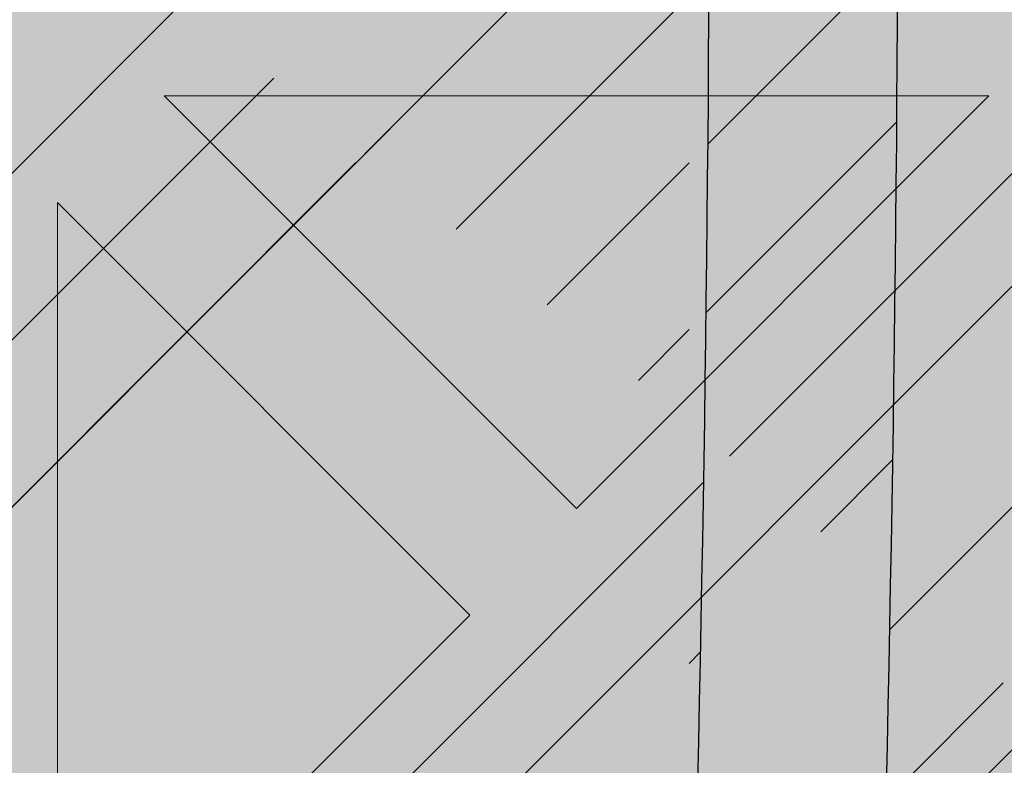
# Model space of a CAD drawing. Units: inches. Extents: x 844 to 2234, y 346 to 1084.
# Tile 11 of 93: x 1122.921 to 1124.585, y 692.442 to 693.702. Entities that reach past the tile are written whole.
import ezdxf

# ---------------------------------------------------------------- set-up
doc = ezdxf.new("R2010")
doc.units = ezdxf.units.IN
doc.header["$MEASUREMENT"] = 0
for name, color, linetype, lineweight in [('A-ANNO-DIMS', 2, 'Continuous', 18), ('furniture', 8, 'Continuous', 18), ('RA-AP-01$0$INT', 35, 'Continuous', 5)]:
    doc.layers.add(name, color=color, linetype=linetype, lineweight=lineweight)
doc.layers.add('RA-AP-01$0$FURN', color=3, linetype='Continuous')
doc.layers.add('RA-AP-01$0$WOOD', color=64, linetype='Continuous')
doc.styles.get("Standard").update_dxf_attribs({"font": 'arial.ttf'})
doc.dimstyles.get("Standard").update_dxf_attribs({"dimtxt": 6, "dimasz": 3, "dimexe": 0.18, "dimexo": 0.0625, "dimgap": 0.09, "dimtad": 0, "dimtih": 1, "dimtoh": 1, "dimdec": 1, "dimzin": 0, "dimdsep": 46, "dimlunit": 3, "dimtxsty": 'Standard', "dimblk": 'ARCHTICK', "dimcen": 0.09, "dimadec": 0, "dimazin": 0, "dimtfac": 1, "dimtdec": 1, "dimtofl": 0, "dimtmove": 0, "dimatfit": 3, "dimfxl": 1, "dimtolj": 1, "dimtzin": 0, "dimarcsym": 0})

# ---------------------------------------------------------------- blocks, each defined once
blk = doc.blocks.new('A$C18D01794')
at = {"layer": 'RA-AP-01$0$INT'}
h = blk.add_hatch(color=256, dxfattribs=at)
h.paths.add_polyline_path([(4.585917135068449, -6.356712009588271), (4.555206456959269, -6.35671200958746), (4.555206456959137, -6.387422687716308), (4.874495778835233, -6.706712009592356), (4.90520645695423, -6.676001331474049)])
h.paths.add_polyline_path([(5.255206456948813, -6.387422687716306), (5.255206456948682, -6.356712009605972), (5.224495778822613, -6.356712009605161), (4.905206456953498, -6.676001331474273), (4.935917135072151, -6.706712009592924)])
h.paths.add_polyline_path([(4.935917135072559, -6.706712009592068), (4.905206456953564, -6.737422687710376), (5.255206456951813, -7.087422687708613), (5.255206456951549, -7.026001331471008)])
h.paths.add_polyline_path([(4.555206456956399, -7.026001331471013), (4.555206456956134, -7.087422687708616), (4.905206456953821, -6.737422687710943), (4.874495778835166, -6.70671200959229)])
h = blk.add_hatch(color=256, dxfattribs=at)
h.paths.add_polyline_path([(4.585917135068448, -6.356712009588273), (4.614201406330596, -6.356712009589021), (4.668846067270487, -6.411356670531338), (4.723490728212344, -6.356712009591912), (4.771774999457151, -6.35671200959319), (4.826419660396886, -6.411356670535356), (4.862780050090322, -6.374996280843536), (4.844495778842715, -6.356712009595112), (4.862780050090411, -6.356712009595595), (4.905206456960182, -6.399138416468211), (4.947632863832445, -6.356712009597838), (4.965917135079675, -6.356712009598322), (4.947632863831759, -6.374996280845421), (4.983993253523576, -6.411356670538857), (5.038637914464627, -6.356712009600247), (5.08692218571208, -6.356712009601523), (5.141566846649976, -6.411356670541852), (5.196211507589851, -6.356712009604411), (5.224495778822615, -6.356712009605161), (4.905206456953975, -6.676001331473793)])
h.paths.add_polyline_path([(4.895206456956031, -6.637717060225675), (4.895206456958921, -6.528427738347902), (4.840561796018589, -6.583072399285802)], flags=16)
h.paths.add_polyline_path([(4.915206456955638, -6.637717060226121), (4.969851117895509, -6.583072399288678), (4.915206456957609, -6.528427738348344)], flags=16)
h.paths.add_polyline_path([(4.826419660395175, -6.568930263661755), (4.881064321335613, -6.514285602723745), (4.771774999456703, -6.514285602720857)], flags=16)
h.paths.add_polyline_path([(4.983993253519558, -6.568930263665262), (5.038637914460456, -6.514285602726792), (4.929348592581548, -6.514285602724816)], flags=16)
h.paths.add_polyline_path([(4.881064321336025, -6.494285602723742), (4.826419660397532, -6.439640941782821), (4.771774999457062, -6.494285602720859)], flags=16)
h.paths.add_polyline_path([(4.929348592582019, -6.494285602724817), (5.038637914460982, -6.494285602726792), (4.983993253522945, -6.439640941786327)], flags=16)
h.paths.add_polyline_path([(4.895206456960191, -6.480143467100443), (4.895206456962115, -6.407422687715913), (4.876922185715016, -6.389138416467584), (4.840561796021581, -6.425498806159401)], flags=16)
h.paths.add_polyline_path([(4.915206456958487, -6.480143467100889), (4.969851117899527, -6.425498806162279), (4.933490728206909, -6.389138416468043), (4.9152064569598, -6.40742268771434)], flags=16)
h.paths.add_polyline_path([(4.757632863832376, -6.480143467096812), (4.812277524772842, -6.425498806158772), (4.757632863834348, -6.370854145217844)], flags=16)
h.paths.add_polyline_path([(4.737632863832376, -6.480143467096286), (4.737632863834348, -6.370854145217375), (4.682988202893906, -6.425498806155385)], flags=16)
h.paths.add_polyline_path([(5.05278005008503, -6.480143467103376), (5.052780050087917, -6.370854145224413), (4.998135389146995, -6.425498806162908)], flags=16)
h.paths.add_polyline_path([(5.072780050085024, -6.480143467103744), (5.127424711025931, -6.42549880616527), (5.072780050087916, -6.370854145224832)], flags=16)
h.paths.add_polyline_path([(4.935917135072783, -6.706712009592292), (5.255206456948811, -6.387422687716309), (5.255206456948932, -6.415706958964177), (5.200561796010279, -6.470351619902839), (5.255206456949403, -6.524996280841948), (5.25520645694961, -6.5732805520894), (5.200561796009787, -6.627925213029239), (5.236922185702417, -6.664285602721864), (5.255206456949919, -6.646001331474357), (5.255206456949998, -6.664285602721898), (5.212780050078687, -6.706712009592262), (5.25520645695036, -6.749138416463932), (5.255206456950438, -6.767422687711313), (5.236922185702424, -6.749138416463297), (5.200561796009796, -6.785498806155928), (5.255206456950753, -6.840143467096874), (5.25520645695096, -6.888427738341682), (5.200561796010322, -6.943072399282328), (5.255206456951428, -6.997717060223427), (5.255206456951547, -7.026001331471006)])
h.paths.add_polyline_path([(5.042988202883395, -6.785498806155427), (5.097632863823085, -6.840143467095101), (5.097632863822622, -6.730854145216193)], flags=16)
h.paths.add_polyline_path([(5.028846067259663, -6.771356670531693), (5.083490728198774, -6.716712009592573), (4.974201406321001, -6.716712009593042)], flags=16)
h.paths.add_polyline_path([(5.117632863823087, -6.840143467095186), (5.172277524762331, -6.785498806155926), (5.11763286382262, -6.730854145216225)], flags=16)
h.paths.add_polyline_path([(5.08349072819877, -6.696712009593886), (5.028846067259652, -6.642067348654775), (4.974201406320998, -6.696712009593438)], flags=16)
h.paths.add_polyline_path([(5.131774999446817, -6.854285602718917), (5.186419660386065, -6.799640941779662), (5.241064321325782, -6.854285602719365)], flags=17)
h.paths.add_polyline_path([(5.131774999446228, -6.716712009592374), (5.186419660386065, -6.771356670532194), (5.222780050079488, -6.734996280838764), (5.204495778832781, -6.716712009592063)], flags=16)
h.paths.add_polyline_path([(5.097632863822613, -6.682569873970264), (5.097632863823061, -6.573280552091354), (5.042988202883383, -6.627925213031044)], flags=16)
h.paths.add_polyline_path([(5.131774999446899, -6.874285602718915), (5.241064321325809, -6.874285602719364), (5.186419660386591, -6.928930263658598)], flags=17)
h.paths.add_polyline_path([(5.131774999446226, -6.696712009594078), (5.204495778830767, -6.696712009594374), (5.22278005007868, -6.67842773834687), (5.186419660386049, -6.642067348654249)], flags=16)
h.paths.add_polyline_path([(5.11763286382262, -6.682569873970225), (5.17227752476232, -6.627925213030515), (5.117632863823064, -6.573280552091267)], flags=16)
h.paths.add_polyline_path([(5.186419660386069, -6.613783077405491), (5.241064321325754, -6.559138416465795), (5.131774999446791, -6.559138416466263)], flags=16)
h.paths.add_polyline_path([(5.131774999446872, -6.539138416466263), (5.24106432132578, -6.539138416465794), (5.186419660386554, -6.484493755526573)], flags=16)
h.paths.add_polyline_path([(5.255206456951811, -7.08742268770861), (5.255206456951895, -7.106712009588038), (4.555206456956052, -7.106712009588038), (4.555206456956136, -7.087422687708617), (4.905206456953973, -6.737422687710788)])
h.paths.add_polyline_path([(4.983993253513404, -6.8444937555241), (4.92934859257295, -6.899138416462108), (5.03863791445186, -6.899138416465014)], flags=16)
h.paths.add_polyline_path([(4.969851117889988, -6.83035161990006), (4.915206456952556, -6.775706958960171), (4.915206456949648, -6.884996280837944)], flags=16)
h.paths.add_polyline_path([(4.929348592572535, -6.919138416462105), (4.983993253511019, -6.973783077403037), (5.038637914451496, -6.919138416465012)], flags=16)
h.paths.add_polyline_path([(5.052780050074912, -6.93328055208906), (4.998135389134438, -6.987925213027088), (5.052780050072919, -7.042569873968025)], flags=16)
h.paths.add_polyline_path([(5.07278005007491, -6.933280552089588), (5.072780050072918, -7.042569873968497), (5.127424711013374, -6.987925213030498)], flags=16)
h.paths.add_polyline_path([(4.89520645695295, -6.775706958959721), (4.840561796013067, -6.830351619897157), (4.895206456950961, -6.884996280837494)], flags=16)
h.paths.add_polyline_path([(4.915206456948365, -6.933280552085403), (4.915206456946434, -7.006001331471951), (4.933490728192729, -7.024285602719066), (4.969851117886972, -6.987925213026453)], flags=16)
h.paths.add_polyline_path([(4.881064321327021, -6.899138416461022), (4.82641966038902, -6.84449375552057), (4.771774999448108, -6.899138416459029)], flags=16)
h.paths.add_polyline_path([(4.895206456950073, -6.933280552084951), (4.840561796009022, -6.987925213023558), (4.876922185700835, -7.024285602716997), (4.895206456948749, -7.006001331469487)], flags=16)
h.paths.add_polyline_path([(4.983993253510392, -7.0020673486505), (4.947632863816944, -7.038427738342319), (4.965917135064043, -7.05671200959023), (5.038637914448995, -7.056712009591555)], flags=16)
h.paths.add_polyline_path([(4.881064321326543, -6.91913841646102), (4.771774999447578, -6.919138416459031), (4.826419660385607, -6.973783077399508)], flags=16)
h.paths.add_polyline_path([(4.905206456946447, -7.014285602717636), (4.862780050074785, -7.056712009588352), (4.947632863816685, -7.056712009589775)], flags=16)
h.paths.add_polyline_path([(5.14156684663679, -7.002067348654549), (5.086922185696452, -7.056712009592438), (5.196211507574223, -7.056712009594425)], flags=16)
h.paths.add_polyline_path([(4.8264196603837, -7.002067348646972), (4.771774999442643, -7.056712009585575), (4.8444957788276, -7.056712009587508), (4.862780050075511, -7.038427738340416)], flags=16)
h.paths.add_polyline_path([(4.812277524760289, -6.98792521302292), (4.757632863822258, -6.933280552082447), (4.757632863819352, -7.042569873961408)], flags=16)
h.paths.add_polyline_path([(4.73763286382226, -6.933280552082079), (4.682988202881349, -6.987925213020536), (4.737632863819352, -7.04256987396099)], flags=16)
h.paths.add_polyline_path([(4.723490728195188, -7.056712009584289), (4.668846067257299, -7.002067348643949), (4.614201406317417, -7.056712009581383)], flags=16)
h.paths.add_polyline_path([(4.597632863829262, -6.706712009592262), (4.555206456957951, -6.664285602721896), (4.555206456958029, -6.646001331474357), (4.573490728205535, -6.664285602721864), (4.609851117898167, -6.627925213029238), (4.555206456958338, -6.573280552089402), (4.555206456958546, -6.524996280841952), (4.60985111789767, -6.470351619902839), (4.555206456959015, -6.415706958964177), (4.555206456959138, -6.387422687716309), (4.874495778835167, -6.70671200959229), (4.5552064569564, -7.026001331471015), (4.555206456956523, -6.997717060223433), (4.609851117897629, -6.94307239928233), (4.555206456956988, -6.888427738341681), (4.555206456957198, -6.840143467096881), (4.609851117898153, -6.78549880615593), (4.573490728205528, -6.749138416463297), (4.555206456957507, -6.76742268771132), (4.555206456957585, -6.749138416463933)])
h.paths.add_polyline_path([(4.712780050085332, -6.730854145216195), (4.712780050084863, -6.840143467095105), (4.767424711024555, -6.785498806155427)], flags=16)
h.paths.add_polyline_path([(4.726922185709173, -6.716712009592573), (4.781566846648288, -6.771356670531693), (4.836211507586949, -6.716712009593043)], flags=16)
h.paths.add_polyline_path([(4.692780050085327, -6.730854145216225), (4.638135389145619, -6.785498806155928), (4.692780050084865, -6.840143467095185)], flags=16)
h.paths.add_polyline_path([(4.726922185709182, -6.696712009593886), (4.836211507586949, -6.696712009593436), (4.7815668466483, -6.642067348654773)], flags=16)
h.paths.add_polyline_path([(4.678637914461726, -6.71671200959237), (4.605917135075169, -6.716712009592063), (4.587632863828464, -6.734996280838766), (4.623993253521887, -6.771356670532195)], flags=16)
h.paths.add_polyline_path([(4.712780050085336, -6.68256987397026), (4.767424711024568, -6.627925213031042), (4.71278005008489, -6.573280552091352)], flags=16)
h.paths.add_polyline_path([(4.678637914461726, -6.696712009594076), (4.623993253521899, -6.642067348654247), (4.587632863829271, -6.67842773834687), (4.605917135077185, -6.696712009594376)], flags=16)
h.paths.add_polyline_path([(4.692780050085336, -6.682569873970228), (4.692780050084889, -6.573280552091267), (4.638135389145632, -6.627925213030515)], flags=16)
h.paths.add_polyline_path([(4.623993253521885, -6.799640941779662), (4.678637914461131, -6.854285602718915), (4.56934859258217, -6.854285602719365)], flags=17)
h.paths.add_polyline_path([(4.623993253521901, -6.613783077405509), (4.678637914461158, -6.559138416466263), (4.569348592582195, -6.559138416465795)], flags=16)
h.paths.add_polyline_path([(4.678637914461051, -6.874285602718915), (4.623993253521361, -6.928930263658598), (4.569348592582143, -6.874285602719364)], flags=17)
h.paths.add_polyline_path([(4.678637914461076, -6.539138416466263), (4.623993253521399, -6.484493755526573), (4.569348592582167, -6.539138416465796)], flags=16)
h = blk.add_hatch(color=256, dxfattribs=at)
h.paths.add_polyline_path([(4.895206456952951, -6.77570695895972), (4.840561796013068, -6.830351619897156), (4.895206456950958, -6.884996280837495)])
h.paths.add_polyline_path([(4.915206456949649, -6.884996280837942), (4.969851117889987, -6.830351619900054), (4.915206456952556, -6.775706958960171)])
h.paths.add_polyline_path([(5.038637914451862, -6.899138416465013), (4.983993253513403, -6.8444937555241), (4.929348592572953, -6.899138416462106)])
h.paths.add_polyline_path([(4.929348592572535, -6.919138416462105), (4.983993253511018, -6.973783077403037), (5.038637914451497, -6.919138416465012)])
h.paths.add_polyline_path([(4.915206456948366, -6.933280552085397), (4.915206456946433, -7.006001331471951), (4.93349072819273, -7.024285602719068), (4.969851117886972, -6.987925213026454)])
h.paths.add_polyline_path([(5.038637914448995, -7.056712009591553), (4.983993253510389, -7.002067348650502), (4.947632863816946, -7.038427738342318), (4.965917135064043, -7.05671200959023)])
h.paths.add_polyline_path([(5.05278005007292, -7.042569873968023), (5.05278005007491, -6.933280552089059), (4.998135389134438, -6.987925213027088)])
h.paths.add_polyline_path([(5.07278005007292, -7.042569873968496), (5.127424711013374, -6.987925213030498), (5.072780050074909, -6.933280552089588)])
h.paths.add_polyline_path([(5.141566846636789, -7.002067348654547), (5.086922185696449, -7.056712009592438), (5.196211507574223, -7.056712009594425)])
h.paths.add_polyline_path([(4.947632863816688, -7.056712009589774), (4.905206456946449, -7.014285602717634), (4.862780050074784, -7.056712009588353)])
h.paths.add_polyline_path([(4.840561796009025, -6.987925213023556), (4.876922185700834, -7.024285602716997), (4.895206456948747, -7.006001331469488), (4.895206456950075, -6.933280552084953)])
h.paths.add_polyline_path([(4.88106432132654, -6.919138416461021), (4.771774999447577, -6.919138416459031), (4.826419660385606, -6.973783077399508)])
h.paths.add_polyline_path([(4.881064321327019, -6.899138416461022), (4.826419660389019, -6.844493755520571), (4.771774999448108, -6.89913841645903)])
h.paths.add_polyline_path([(4.757632863819352, -7.042569873961409), (4.812277524760284, -6.987925213022922), (4.757632863822259, -6.933280552082447)])
h.paths.add_polyline_path([(4.8264196603837, -7.002067348646974), (4.771774999442646, -7.056712009585575), (4.844495778827599, -7.05671200958751), (4.862780050075512, -7.038427738340417)])
h.paths.add_polyline_path([(4.737632863819352, -7.042569873960988), (4.737632863822258, -6.933280552082078), (4.682988202881349, -6.987925213020538)])
h.paths.add_polyline_path([(4.668846067257299, -7.002067348643952), (4.61420140631742, -7.056712009581384), (4.723490728195189, -7.056712009584292)])
for p, q in [((4.935917135072783, -6.706712009592292), (5.255206456951548, -7.026001331471007)), ((4.905206456953975, -6.737422687710788), (5.255206456951811, -7.087422687708611)), ((4.915206456952556, -6.775706958960171), (4.969851117889986, -6.830351619900053)), ((4.915206456949648, -6.884996280837942), (4.915206456952556, -6.775706958960171)), ((4.915206456949651, -6.88499628083794), (4.969851117889986, -6.830351619900053)), ((4.929348592572952, -6.899138416462106), (4.983993253513403, -6.844493755524101)), ((4.983993253513404, -6.844493755524103), (5.038637914451862, -6.899138416465012)), ((5.038637914451862, -6.899138416465012), (4.929348592572952, -6.899138416462106))]:
    blk.add_line(p, q, dxfattribs=at)
blk = doc.blocks.new('A$C32926AE1')
at = {"layer": 'RA-AP-01$0$FURN'}
h = blk.add_hatch(dxfattribs=at)
h.set_pattern_fill('ANSI31', color=256, scale=0.1, style=0)
h.set_pattern_definition([(45, (0, 0), (-0.0088388347648318, 0.0088388347648318), [])])
edge = h.paths.add_edge_path(flags=16)
edge.add_arc((4.904771284329206, 4.246793130718756), 0.2603971832811541, 75.22398030683196, 104.7760196931204)
edge.add_arc((4.904771284329206, 4.246793130718756), 0.2603971832811541, 75.223980306832, 104.77601969312039, ccw=False)
edge = h.paths.add_edge_path(flags=16)
edge.add_arc((4.904771284329206, 4.067062675376612), 0.2603971832811541, 255.2239803068796, 284.776019693168)
edge.add_arc((4.904771284329206, 4.067062675376612), 0.2603971832811541, 255.22398030687958, 284.77601969316805, ccw=False)
edge = h.paths.add_edge_path(flags=0)
edge.add_arc((4.904771284329206, 4.067062675376612), 0.2603971832811541, 255.2239803068796, 284.776019693168)
edge.add_arc((4.904771284329206, 4.067062675376612), 0.2603971832811541, 255.22398030687958, 284.77601969316805, ccw=False)
edge = h.paths.add_edge_path(flags=0)
edge.add_arc((4.904771284329206, 4.067062675376612), 0.2603971832811541, 255.2239803068796, 284.776019693168)
edge.add_arc((4.904771284329206, 4.067062675376612), 0.2603971832811541, 255.22398030687958, 284.77601969316805, ccw=False)
edge = h.paths.add_edge_path()
edge.add_arc((4.604388392048174, 4.588829985554312), 0.1599999999999918, 342.3781640246255, 354.4317409793762)
edge.add_arc((5.090145208887507, 4.43216705527679), 0.3503971832811637, 162.0091218307731, 180.3186872093483)
edge.add_arc((5.205154176610243, 4.588829985554953), 0.1599999999999917, 185.5682590208461, 197.6218359767349)
edge.add_arc((4.904771284329229, 4.246793130718735), 0.3503971832811761, 72.00912183053516, 107.9908781690354)
edge.add_arc((9.535952835716557, 4.28682295566602), 4.798342501046485, 178.2875002453811, 181.5576802719453)
edge.add_arc((4.719397359771122, 4.43216705527679), 0.3503971832811637, 359.6813127906516, 377.9908781692269)
edge.add_arc((9.535967292294904, 4.286822350292874), 4.778371420254705, 178.2965938931842, 181.5667745797229)
edge.add_arc((4.719397359771122, 4.43216705527679), 0.3303971832811637, 359.6813127906516, 377.9908781692269)
edge.add_arc((0.2735752763637294, 4.286822350292874), 4.7783714202547, 358.4332254202771, 361.7034061068158)
edge.add_arc((5.061434214606998, 4.732549947558029), 0.1600000000000254, 252.3781640250584, 264.4317409792362)
edge.add_arc((4.748108354051257, 4.732549947558012), 0.1600000000000541, 275.5682590208426, 287.6218359759532)
edge.add_arc((4.604388392048115, 4.588829985554317), 0.1800000000000505, 342.3567572500182, 349.3735009646207)
edge.add_arc((5.205154176610254, 4.588829985554976), 0.1800000000000069, 190.6264990356027, 197.6432427513933)
edge.add_arc((5.061434214607106, 4.732549947558013), 0.1800000000000424, 252.3567572496606, 259.3735009644582)
edge.add_arc((4.904771284329208, 4.246793130718737), 0.3303971832811676, 71.99844483668534, 108.0015551637021)
edge.add_arc((4.748108354051414, 4.732549947558045), 0.1800000000000547, 280.6264990355479, 287.6432427495938)
edge.add_arc((5.090145208887514, 4.432167055276789), 0.2803971832811691, 162.8706300666893, 180.816523289902)
edge.add_arc((4.719397359771136, 4.432167055276689), 0.2803971832811534, 359.183476710103, 377.1293699333214)
edge.add_arc((4.904771284329222, 4.246793130718737), 0.2803971832811769, 72.87063006672916, 107.1293699332334)
edge.add_arc((5.090145208887522, 4.432167055276788), 0.2603971832811776, 165.2239803068007, 180.9953123810312)
edge.add_arc((4.719397359771141, 4.432167055276699), 0.2603971832811458, 359.0046876189768, 374.7760196932087)
edge.add_arc((5.090145208887507, 4.43216705527679), 0.3303971832811637, 162.0091218307731, 180.3186872093483)
edge.add_arc((9.53595427642584, 4.285015535491528), 4.728345371032053, 178.265043920078, 181.5679956281801)
edge.add_arc((0.2735882922327999, 4.285015535491582), 4.728345371032045, 358.4320043718193, 361.7349560799204)
edge.add_arc((9.535953591267507, 4.284458026472751), 4.708343996644348, 178.2573054306777, 181.5704995759608)
edge.add_arc((0.273588977391114, 4.284458026472785), 4.708343996644358, 358.4295004240388, 361.7426945693213)
edge.add_arc((0.2735889773911131, 4.029397779622582), 4.708343996644359, 358.2573054306787, 361.5704995759613)
edge.add_arc((9.535953591267518, 4.029397779622618), 4.708343996644359, 178.4295004240391, 181.7426945693223)
edge.add_arc((0.2735882922327901, 4.028840270603786), 4.728345371032054, 358.2650439200796, 361.5679956281808)
edge.add_arc((9.53595427642584, 4.028840270603841), 4.728345371032054, 178.4320043718199, 181.7349560799219)
edge.add_arc((0.2735752763637302, 4.027033455802493), 4.778371420254699, 358.2965938931842, 361.5667745797229)
edge.add_arc((4.719397359771122, 3.881688750818578), 0.3303971832811637, 342.0091218307731, 360.3186872093484)
edge.add_arc((5.090145208887507, 3.881688750818578), 0.3303971832811637, 179.6813127906516, 197.9908781692269)
edge.add_arc((9.535967292294904, 4.027033455802493), 4.778371420254705, 178.433225420277, 181.7034061068158)
edge.add_arc((4.719397359771122, 3.881688750818578), 0.3503971832811637, 342.0091218307731, 360.3186872093484)
edge.add_arc((9.53595283571655, 4.027032850429349), 4.79834250104648, 178.4423197280546, 181.7124997546188)
edge.add_arc((4.719397359771141, 3.881688750818669), 0.2603971832811458, 345.2239803067913, 360.9953123810232)
edge.add_arc((5.090145208887522, 3.88168875081858), 0.2603971832811776, 179.0046876189687, 194.7760196931993)
edge.add_arc((4.904771284329222, 4.067062675376631), 0.2803971832811769, 252.8706300667665, 287.1293699332708)
edge.add_arc((4.719397359771136, 3.881688750818678), 0.2803971832811534, 342.8706300666787, 360.8165232898969)
edge.add_arc((5.090145208887514, 3.881688750818579), 0.2803971832811691, 179.183476710098, 197.1293699333106)
edge.add_arc((4.748108354051414, 3.581305858537323), 0.1800000000000547, 72.3567572504062, 79.37350096445199)
edge.add_arc((4.904771284329208, 4.067062675376631), 0.3303971832811676, 251.9984448362979, 288.0015551633146)
edge.add_arc((5.061434214607106, 3.581305858537355), 0.1800000000000424, 100.6264990355418, 107.6432427503394)
edge.add_arc((5.205154176610254, 3.725025820540392), 0.1800000000000069, 162.3567572486066, 169.3735009643972)
edge.add_arc((4.604388392048115, 3.725025820541051), 0.1800000000000505, 10.62649903537925, 17.64324274998182)
edge.add_arc((4.748108354051257, 3.581305858537356), 0.1600000000000541, 72.37816402404681, 84.43174097915735)
edge.add_arc((4.904771284329229, 4.067062675376632), 0.3503971832811761, 252.0091218309645, 287.9908781694648)
edge.add_arc((5.061434214606998, 3.581305858537339), 0.1600000000000254, 95.56825902076373, 107.6218359749416)
edge.add_arc((5.205154176610243, 3.725025820540414), 0.1599999999999917, 162.3781640232651, 174.4317409791539)
edge.add_arc((5.090145208887507, 3.881688750818578), 0.3503971832811637, 179.6813127906516, 197.9908781692269)
edge.add_arc((4.604388392048174, 3.725025820541056), 0.1599999999999918, 5.568259020623824, 17.62183597537444)
edge.add_arc((0.2735897329420762, 4.28682295566602), 4.798342501046482, 358.4423197280547, 361.7124997546188)
edge.add_arc((0.2735897329420691, 4.027032850429348), 4.798342501046489, 358.2875002453812, 361.5576802719453)
at = {"layer": 'RA-AP-01$0$WOOD'}
h = blk.add_hatch(color=256, dxfattribs=at)
h.dxf.hatch_style = 1
h.paths.add_polyline_path([(5.157430609644524, 4.573483066760929, -0.1009492694046607), (5.155401577623758, 4.593365984175333, -0.1842662638101597), (5.172249623284174, 4.638795604568598, 0.2056608120311276), (5.179560981299304, 4.661316324430096, 0.3614336704623542), (5.134352340494423, 4.706524965234944, 0.2056608120311297), (5.111831620632933, 4.699213607219793, -0.1842662638101113), (5.066402000239693, 4.682365561559342, -0.1055311479399994), (5.045656153913092, 4.68467289944697, 0.1567636581983829), (4.763886414745334, 4.684672899446966, -0.1055311479399895), (4.743140568418733, 4.68236556155934, -0.1842662638100833), (4.6977109480255, 4.69921360721979, 0.2056608120302612), (4.675190228164109, 4.706524965234949, 0.3614336704708441), (4.629981587358889, 4.66131632442871, 0.2056608120245944), (4.637292945374126, 4.638795604567974, -0.1842662638101024), (4.654140991034615, 4.59336598417475, -0.1009492694055169), (4.652111959013835, 4.573483066760181, 0.021410119221476), (4.629748025606143, 4.156712009541676, 0.0214101192214795), (4.652111959013809, 3.739940952323101, -0.1009492694059586), (4.654140991034615, 3.720058034908448, -0.1842662638100975), (4.637292945374126, 3.674628414515226, 0.2056608120245705), (4.629981587358889, 3.652107694654492, 0.3614336704708879), (4.675190228164113, 3.606899053848249, 0.2056608120302384), (4.697710948025501, 3.614210411863408, -0.1842662638100995), (4.743140568418738, 3.63105845752386, -0.1055311479402541), (4.763886414745388, 3.628751119636215, 0.1567636581983776), (5.045656153913137, 3.628751119636244, -0.1055311479397538), (5.066402000239692, 3.631058457523857, -0.1842662638101067), (5.111831620632931, 3.614210411863407, 0.2056608120310924), (5.134352340494417, 3.606899053848256, 0.3614336704624001), (5.179560981299307, 3.652107694653103, 0.2056608120311314), (5.172249623284175, 3.6746284145146, -0.1842662638101402), (5.155401577623758, 3.72005803490786, -0.1009492694051366), (5.15743060964455, 3.739940952322354, 0.0214101192215073), (5.179794543052287, 4.156712009541468, 0.0214101192215252)])
h.paths.add_polyline_path([(4.639748609479751, 4.156712009541513, 0.0213537860821624), (4.661970494867118, 3.741887061152232, -0.094075836301374), (4.664143710413708, 3.7196126951003, -0.1824818158568985), (4.644813765429836, 3.668037719127816, 0.2056608120245319), (4.639939526753007, 3.653023905887301, 0.3614336704710246), (4.676106439397173, 3.616856993242342, 0.2056608120302234), (4.691120252638095, 3.621731231919122, -0.1824818158602558), (4.742695228611606, 3.641061176902986, -0.1029891339458722), (4.766991894714349, 3.638256818950944, 0.156709409989566), (5.042550673941472, 3.638256818950105, -0.102989133958497), (5.066847340047078, 3.641061176902949, -0.1824818158594995), (5.118422316020358, 3.621731231919103, 0.2056608120311416), (5.133436129261316, 3.616856993242346, 0.3614336704621468), (5.169603041905217, 3.653023905886178, 0.2056608120310986), (5.164728803228477, 3.668037719127177, -0.1824818158565612), (5.145398858244737, 3.719612695099578, -0.0940758363009313), (5.147572073791232, 3.741887061151398, 0.0213537860822023), (5.169793959178681, 4.156712009541451, 0.0213537860822226), (5.147572073791203, 4.571536957931898, -0.0940758363005034), (5.145398858244737, 4.59381132398362, -0.1824818158565587), (5.164728803228476, 4.645386299956021, 0.2056608120311045), (5.169603041905216, 4.66040011319702, 0.3614336704621845), (5.133436129261313, 4.696567025840856, 0.2056608120310773), (5.118422316020359, 4.691692787164098, -0.182481815859508), (5.066847340047078, 4.67236284218025, -0.1029891339584606), (5.04255067394148, 4.675167200133092, 0.156709409989566), (4.766991894714357, 4.675167200132257, -0.1029891339458842), (4.742695228611611, 4.672362842180213, -0.1824818158602725), (4.691120252638095, 4.691692787164077, 0.2056608120302152), (4.676106439397174, 4.696567025840858, 0.3614336704710363), (4.639939526753005, 4.660400113195899, 0.2056608120245495), (4.644813765429837, 4.645386299955384, -0.1824818158568934), (4.664143710413708, 4.593811323982902, -0.0940758363009187), (4.661970494867149, 4.571536957931074, 0.021353786082177)], flags=16)
h.paths.add_polyline_path([(5.129794543052235, 4.432167055276933, -0.0141661062790638), (5.130152669293814, 4.156927903047693, -0.0141661062790647), (5.129794543052234, 3.881688750818433, -0.0785247771143638), (5.10979738006795, 3.755143611847103, 0.0945969212073497), (5.105408519571111, 3.717898134952927, 0.1043170707844957), (5.116074640131521, 3.670385395016088, 0.1043170707864965), (5.068561900193738, 3.681051515576561, 0.09459692119553), (5.031316423304057, 3.676662655080835, -0.1580239521427272), (4.778226145355827, 3.676662655080367, 0.0945969211986668), (4.740980668464973, 3.681051515576592, 0.1043170707882822), (4.693467928526415, 3.670385395015844, 0.1043170707867916), (4.704134049087309, 3.717898134953662, 0.0945969211972894), (4.69974518859162, 3.755143611844042, -0.0785247771163196), (4.679748025606343, 3.881688750818406, -0.0141661062790663), (4.679389899364763, 4.156927903047693, -0.0141661062790672), (4.679748025606343, 4.432167055276998, -0.0785247771163064), (4.699745188591625, 4.55871219425134, 0.094596921197333), (4.704134049087308, 4.595957671141738, 0.1043170707867205), (4.693467928526416, 4.643470411079523, 0.1043170707882628), (4.740980668464965, 4.632804290518776, 0.0945969211988114), (4.778226145355874, 4.637193151015016, -0.158023952142669), (5.031316423304015, 4.637193151014546, 0.0945969211956361), (5.068561900193736, 4.632804290518806, 0.1043170707864979), (5.11607464013152, 4.643470411079278, 0.1043170707844617), (5.105408519571112, 4.595957671142455, 0.0945969212074597), (5.109797380067959, 4.558712194248236, -0.0785247771143467)], flags=0)
h.paths.add_polyline_path([(5.119794532311105, 4.432259799204851, -0.0142000800617244), (5.120156169157484, 4.156927903047701, -0.0142000800617277), (5.119794532311105, 3.881596006890482, -0.0784894509520253), (5.100273383573699, 3.758192358677797, 0.0940138827242913), (5.095413455884425, 3.717477693979438, 0.0606271852308753), (5.099615656341024, 3.686844378806616, 0.0606271852322524), (5.068982341167493, 3.691046579263239, 0.0940138827010453), (5.028267676478798, 3.686186651576848, -0.1580706864508061), (4.781274892180912, 3.686186651576435, 0.0940138827026903), (4.740560227491556, 3.691046579263279, 0.0606271852339895), (4.709926912317155, 3.686844378806508, 0.0606271852329405), (4.714129112773991, 3.717477693980356, 0.094013882701304), (4.709269185087677, 3.758192358669163, -0.0784894509577193), (4.689748036347473, 3.881596006890469, -0.014200080061729), (4.689386399501094, 4.156927903047709, -0.0142000800617217), (4.689748036347473, 4.432259799204808, -0.078489450957724), (4.709269185087651, 4.555663447426125, 0.0940138827014585), (4.714129112773992, 4.596378112114996, 0.0606271852329731), (4.709926912317154, 4.62701142728886, 0.0606271852340196), (4.74056022749157, 4.622809226832087, 0.0940138827024997), (4.781274892180847, 4.627669154518912, -0.1580706864508359), (5.028267676478777, 4.627669154518526, 0.0940138827010946), (5.068982341167492, 4.622809226832129, 0.060627185232254), (5.099615656341024, 4.627011427288751, 0.0606271852308727), (5.095413455884425, 4.59637811211593, 0.0940138827241088), (5.100273383573675, 4.555663447417647, -0.0784894509520978)], flags=0)
h.paths.add_polyline_path([(5.06978912287499, 4.430218106756144, -0.014241683694547), (5.070173729147532, 4.156927903047672, -0.0142416836945458), (5.06978912287499, 3.883637699339223, -0.0800609523125196), (5.052662118612511, 3.773463122773442, 0.0526421978001116), (5.04590916754064, 3.740550867606997, 0.0526421977992423), (5.012996912374707, 3.73379791653534, -0.1583028414718258), (4.796545656286308, 3.73379791653451, 0.0526421978034211), (4.763633401117837, 3.740550867607021, 0.0526421978018622), (4.756880450045755, 3.773463122774558, -0.0800609523117106), (4.739753445783639, 3.883637699339268, -0.0142416836945435), (4.739368839511098, 4.156927903047671, -0.0142416836945477), (4.739753445783639, 4.430218106756155, -0.0800609523116345), (4.75688045004574, 4.540392683320762, 0.052642197801941), (4.763633401117837, 4.573304938488346, 0.0526421978035071), (4.796545656286361, 4.580057889560873, -0.1583028414717561), (5.012996912374669, 4.580057889560039, 0.0526421977993048), (5.04590916754064, 4.57330493848837, 0.0526421978002057), (5.052662118612529, 4.540392683321868, -0.080060952312477)], flags=0)
h.paths.add_polyline_path([(5.049789715110557, 4.43038092723357, -0.0143097550741839), (5.05018085590259, 4.156927903047715, -0.0143097550741854), (5.049789715110558, 3.883474878861827, -0.0800685599149176), (5.03362098255317, 3.779581877367999, 0.0306258898956367), (5.028241146483733, 3.758218888663947, 0.0306258898977031), (5.006878157778253, 3.75283905259408, -0.1583983521624096), (4.802664410878162, 3.752839052594731, 0.0306258898946014), (4.781301422174808, 3.758218888663924, 0.0306258898967912), (4.775921586105202, 3.779581877368794, -0.080068559914251), (4.759752853548071, 3.883474878861786, -0.0143097550741854), (4.759361712756037, 4.156927903047671, -0.0143097550741854), (4.759752853548071, 4.430380927233557, -0.0800685599142479), (4.775921586105193, 4.534273928726546, 0.0306258898968306), (4.781301422174808, 4.555636917431444, 0.0306258898945754), (4.802664410878143, 4.561016753500631, -0.1583983521624168), (5.006878157778244, 4.561016753501291, 0.0306258898977177), (5.028241146483733, 4.555636917431421, 0.0306258898958182), (5.03362098255321, 4.534273928727244, -0.080068559914796)], flags=0)
h.paths.add_polyline_path([(4.999766070382627, 4.428171244713864, -0.0143443147609634), (5.000198441819402, 4.156927903047689, -0.0143443147609612), (4.999766070382627, 3.885684561381556, -0.0784641635803329), (4.987356730658798, 3.799103304488872, -0.1506053783831347), (4.822185837999821, 3.79910330448882, -0.0784641635803318), (4.809776498276007, 3.885684561381509, -0.014344314760963), (4.809344126839227, 4.156927903047677, -0.0143443147609645), (4.809776498276007, 4.428171244713873, -0.0784641635803192), (4.822185837999822, 4.514752501606549, -0.1506053783831338), (4.987356730658798, 4.514752501606494, -0.078464163580285)], flags=0)
h.paths.add_polyline_path([(4.979755254238824, 4.42764379880488, -0.0143772539198268), (4.980205517789977, 4.156927903047693, -0.0143772539198275), (4.979755254238824, 3.886212007290489, -0.0689242507424422), (4.971183264704897, 3.815276770442801, -0.1296645318904179), (4.838359303953726, 3.815276770442746, -0.0689242507424186), (4.829787314419809, 3.886212007290419, -0.0143772539198292), (4.829337050868653, 4.156927903047653, -0.0143772539198325), (4.829787314419809, 4.427643798804946, -0.0689242507424211), (4.838359303953725, 4.498579035652621, -0.1296645318904187), (4.971183264704897, 4.498579035652565, -0.0689242507424401)], flags=0)
h = blk.add_hatch(color=256, dxfattribs=at)
h.dxf.hatch_style = 1
h.paths.add_polyline_path([(5.145398858244737, 4.59381132398362, -0.1824818158565616), (5.164728803228476, 4.645386299956021, 0.2056608120311045), (5.169603041905216, 4.66040011319702, 0.3614336704621845), (5.133436129261313, 4.696567025840856, 0.2056608120310773), (5.118422316020359, 4.691692787164098, -0.182481815859508), (5.066847340047078, 4.67236284218025, -0.1029891339584606), (5.04255067394148, 4.675167200133092, 0.156709409989566), (4.766991894714357, 4.675167200132257, -0.1029891339458842), (4.742695228611611, 4.672362842180213, -0.1824818158602725), (4.691120252638095, 4.691692787164077, 0.2056608120302152), (4.676106439397174, 4.696567025840858, 0.3614336704710363), (4.639939526753005, 4.660400113195899, 0.2056608120245495), (4.644813765429837, 4.645386299955384, -0.1824818158568934), (4.664143710413708, 4.593811323982902, -0.0940758363009187), (4.661970494867149, 4.571536957931074, 0.0213537860821772), (4.639748609479751, 4.156712009541507, 0.0213537860821625), (4.661970494867119, 3.741887061152226, -0.0940758363013071), (4.664143710413708, 3.719612695100309, -0.1824818158569294), (4.644813765429836, 3.668037719127816, 0.2056608120245319), (4.639939526753007, 3.653023905887301, 0.3614336704710246), (4.676106439397173, 3.616856993242342, 0.2056608120302234), (4.691120252638095, 3.621731231919122, -0.1824818158602558), (4.742695228611606, 3.641061176902986, -0.1029891339458722), (4.766991894714349, 3.638256818950944, 0.156709409989566), (5.042550673941472, 3.638256818950105, -0.102989133958497), (5.066847340047078, 3.641061176902949, -0.1824818158594995), (5.118422316020358, 3.621731231919103, 0.2056608120311416), (5.133436129261316, 3.616856993242346, 0.3614336704621468), (5.169603041905217, 3.653023905886178, 0.2056608120310986), (5.164728803228477, 3.668037719127177, -0.1824818158565612), (5.145398858244737, 3.719612695099578, -0.0940758363009313), (5.147572073791232, 3.741887061151398, 0.0213537860822023), (5.169793959178681, 4.156712009541451, 0.0213537860822226), (5.147572073791203, 4.571536957931898, -0.0940758363004996)])
h.paths.add_polyline_path([(5.109797380067958, 4.55871219424824, -0.0785247771143472), (5.129794543052234, 4.432167055276936, -0.0141661062790644), (5.130152669293814, 4.156927903047685, -0.014166106279066), (5.129794543052234, 3.881688750818401, -0.0785247771143517), (5.109797380067946, 3.755143611847092, 0.0945969212073132), (5.105408519571111, 3.717898134952929, 0.1043170707844995), (5.116074640131521, 3.670385395016088, 0.1043170707864965), (5.068561900193738, 3.681051515576561, 0.09459692119553), (5.031316423304057, 3.676662655080835, -0.1580239521427272), (4.778226145355827, 3.676662655080367, 0.0945969211986668), (4.740980668464973, 3.681051515576592, 0.1043170707882822), (4.693467928526415, 3.670385395015844, 0.1043170707867916), (4.704134049087309, 3.717898134953662, 0.0945969211972894), (4.69974518859162, 3.755143611844042, -0.0785247771163196), (4.679748025606343, 3.881688750818406, -0.0141661062790663), (4.679389899364763, 4.156927903047693, -0.0141661062790672), (4.679748025606343, 4.432167055276998, -0.0785247771163064), (4.699745188591625, 4.55871219425134, 0.094596921197333), (4.704134049087308, 4.595957671141738, 0.1043170707867205), (4.693467928526416, 4.643470411079523, 0.1043170707882628), (4.740980668464965, 4.632804290518776, 0.0945969211988114), (4.778226145355874, 4.637193151015016, -0.158023952142669), (5.031316423304015, 4.637193151014546, 0.0945969211956361), (5.068561900193736, 4.632804290518806, 0.1043170707864979), (5.11607464013152, 4.643470411079278, 0.1043170707844617), (5.105408519571112, 4.595957671142455, 0.0945969212074504)], flags=16)
h.paths.add_polyline_path([(5.100273383573655, 4.55566344741771, -0.0784894509521388), (5.119794532311105, 4.432259799204852, -0.0142000800617252), (5.120156169157484, 4.156927903047686, -0.014200080061726), (5.119794532311105, 3.881596006890502, -0.0784894509520446), (5.100273383573696, 3.758192358677786, 0.0940138827242721), (5.095413455884425, 3.717477693979436, 0.0606271852308692), (5.099615656341024, 3.686844378806616, 0.0606271852322522), (5.068982341167493, 3.691046579263239, 0.0940138827010453), (5.028267676478798, 3.686186651576848, -0.1580706864508061), (4.781274892180912, 3.686186651576435, 0.0940138827026903), (4.740560227491556, 3.691046579263279, 0.0606271852339895), (4.709926912317155, 3.686844378806508, 0.0606271852329405), (4.714129112773991, 3.717477693980356, 0.094013882701304), (4.709269185087677, 3.758192358669163, -0.0784894509577193), (4.689748036347473, 3.881596006890469, -0.014200080061729), (4.689386399501094, 4.156927903047709, -0.0142000800617217), (4.689748036347473, 4.432259799204808, -0.078489450957724), (4.709269185087651, 4.555663447426125, 0.0940138827014585), (4.714129112773992, 4.596378112114996, 0.0606271852329731), (4.709926912317154, 4.62701142728886, 0.0606271852340196), (4.74056022749157, 4.622809226832087, 0.0940138827024997), (4.781274892180847, 4.627669154518912, -0.1580706864508359), (5.028267676478777, 4.627669154518526, 0.0940138827010946), (5.068982341167492, 4.622809226832129, 0.060627185232254), (5.099615656341024, 4.627011427288751, 0.0606271852308727), (5.095413455884425, 4.59637811211593, 0.094013882723957)], flags=0)
h.paths.add_polyline_path([(5.04590916754064, 4.57330493848837, 0.0526421978002057), (5.052662118612529, 4.540392683321868, -0.0800609523124783), (5.06978912287499, 4.430218106756142, -0.0142416836945469), (5.070173729147532, 4.156927903047672, -0.0142416836945458), (5.06978912287499, 3.883637699339223, -0.0800609523125196), (5.052662118612511, 3.773463122773442, 0.0526421978001116), (5.04590916754064, 3.740550867606997, 0.0526421977992423), (5.012996912374707, 3.73379791653534, -0.1583028414718258), (4.796545656286308, 3.73379791653451, 0.0526421978034211), (4.763633401117837, 3.740550867607021, 0.0526421978018622), (4.756880450045755, 3.773463122774558, -0.0800609523117106), (4.739753445783639, 3.883637699339268, -0.0142416836945435), (4.739368839511098, 4.156927903047671, -0.0142416836945477), (4.739753445783639, 4.430218106756155, -0.0800609523116345), (4.75688045004574, 4.540392683320762, 0.052642197801941), (4.763633401117837, 4.573304938488346, 0.0526421978035071), (4.796545656286361, 4.580057889560873, -0.1583028414717561), (5.012996912374669, 4.580057889560039, 0.0526421977993048)], flags=0)
h.paths.add_polyline_path([(5.028241146483733, 4.555636917431422, 0.0306258898956949), (5.033620982553182, 4.534273928727329, -0.0800685599148649), (5.049789715110557, 4.430380927233569, -0.0143097550741839), (5.05018085590259, 4.156927903047715, -0.0143097550741854), (5.049789715110558, 3.883474878861827, -0.0800685599149176), (5.03362098255317, 3.779581877367999, 0.0306258898956367), (5.028241146483733, 3.758218888663947, 0.0306258898977031), (5.006878157778253, 3.75283905259408, -0.1583983521624096), (4.802664410878162, 3.752839052594731, 0.0306258898946014), (4.781301422174808, 3.758218888663924, 0.0306258898967912), (4.775921586105202, 3.779581877368794, -0.080068559914251), (4.759752853548071, 3.883474878861786, -0.0143097550741854), (4.759361712756037, 4.156927903047671, -0.0143097550741854), (4.759752853548071, 4.430380927233557, -0.0800685599142479), (4.775921586105193, 4.534273928726546, 0.0306258898968306), (4.781301422174808, 4.555636917431444, 0.0306258898945754), (4.802664410878143, 4.561016753500631, -0.1583983521624168), (5.006878157778244, 4.561016753501291, 0.0306258898977174)], flags=0)
h.paths.add_polyline_path([(4.987356730658798, 4.514752501606494, -0.0784641635803018), (4.999766070382627, 4.428171244713845, -0.0143443147609637), (5.000198441819402, 4.156927903047665, -0.0143443147609622), (4.999766070382628, 3.885684561381514, -0.0784641635802952), (4.987356730658797, 3.799103304488872, -0.1506053783831338), (4.822185837999821, 3.799103304488819, -0.0784641635803342), (4.809776498276007, 3.885684561381512, -0.0143443147609628), (4.809344126839227, 4.156927903047676, -0.0143443147609646), (4.809776498276007, 4.428171244713873, -0.0784641635803192), (4.822185837999822, 4.514752501606549, -0.1506053783831338)], flags=0)
h.paths.add_polyline_path([(4.971183264704897, 4.498579035652566, -0.0689242507424384), (4.979755254238824, 4.427643798804883, -0.0143772539198276), (4.980205517789977, 4.15692790304768, -0.0143772539198258), (4.979755254238823, 3.88621200729051, -0.0689242507424628), (4.971183264704897, 3.815276770442801, -0.129664531890417), (4.838359303953726, 3.815276770442746, -0.0689242507424186), (4.829787314419809, 3.886212007290419, -0.0143772539198292), (4.829337050868653, 4.156927903047653, -0.0143772539198325), (4.829787314419809, 4.427643798804946, -0.0689242507424211), (4.838359303953725, 4.498579035652621, -0.1296645318904187)], flags=0)
h = blk.add_hatch(dxfattribs=at)
h.set_pattern_fill('ANSI31', color=256, scale=0.05, style=0)
h.set_pattern_definition([(45, (0, 0), (-0.0044194173824159, 0.0044194173824159), [])])
h.paths.add_polyline_path([(5.130152669293814, 4.156927903047704, 0.0141661062790657), (5.129794543052234, 4.432167055276982, 0.0777827904001433), (5.110168979996553, 4.557559993161921, -0.0976515123401879), (5.105408519571111, 4.595957671142454, -0.1043170707844687), (5.116074640131522, 4.64347041107928), (5.099615656341024, 4.627011427288751, 0.0606271852308727), (5.095413455884425, 4.59637811211593, 0.0940138827241088), (5.100273383573675, 4.555663447417647, -0.0784894509520972), (5.119794532311105, 4.432259799204852, -0.0142000800617252), (5.120156169157484, 4.156927903047686, -0.014200080061726), (5.119794532311105, 3.881596006890502, -0.0784894509520446), (5.100273383573696, 3.758192358677786, 0.0940138827242721), (5.095413455884425, 3.717477693979436, 0.0606271852308692), (5.099615656341024, 3.686844378806616), (5.116074640131519, 3.67038539501609, -0.1043170707844594), (5.105408519571112, 3.717898134952912, -0.0976515123401594), (5.11016897999655, 3.756295812933435, 0.0777827904001654), (5.129794543052234, 3.881688750818409, 0.0141661062790665)])
h.paths.add_polyline_path([(5.030164222210597, 3.676291055149937, -0.0976515123472002), (5.068561900193739, 3.681051515576561, -0.1043170707864927), (5.116074640131521, 3.670385395016088), (5.099615656341024, 3.686844378806616, 0.0606271852322522), (5.068982341167493, 3.691046579263239, 0.0940138827010453), (5.028267676478798, 3.686186651576848, -0.1580706864508061), (4.781274892180912, 3.686186651576435, 0.0940138827026903), (4.740560227491556, 3.691046579263279, 0.0606271852339913), (4.709926912317154, 3.686844378806508), (4.693467928526416, 3.670385395015845, -0.1043170707882796), (4.740980668464973, 3.681051515576592, -0.0976515123427246), (4.779378346446416, 3.676291055150394, 0.156512506893803)])
h.paths.add_polyline_path([(4.689748036347473, 3.881596006890472, -0.014200080061729), (4.689386399501094, 4.156927903047712, -0.0142000800617195), (4.689748036347473, 4.432259799204768, -0.078489450957742), (4.709269185087648, 4.555663447426114, 0.0940138827014821), (4.714129112773992, 4.596378112114995, 0.0606271852329748), (4.709926912317154, 4.62701142728886), (4.693467928526414, 4.643470411079524, -0.1043170707867939), (4.704134049087309, 4.595957671141706, -0.09765151234893), (4.699373588660725, 4.557559993157876, 0.0777827903975372), (4.679748025606343, 4.432167055276987, 0.0141661062790675), (4.679389899364763, 4.156927903047675, 0.0141661062790641), (4.679748025606343, 3.88168875081843, 0.0777827903975637), (4.699373588660724, 3.756295812937497, -0.0976515123490278), (4.704134049087308, 3.717898134953629, -0.1043170707867196), (4.693467928526416, 3.670385395015845), (4.709926912317155, 3.686844378806508, 0.0606271852329413), (4.714129112773991, 3.717477693980357, 0.0940138827013084), (4.709269185087676, 3.758192358669166, -0.0784894509577192)])
h.paths.add_polyline_path([(4.779378346446434, 4.63756475094498, -0.0976515123427943), (4.740980668464964, 4.632804290518776, -0.1043170707882609), (4.693467928526416, 4.643470411079523), (4.709926912317154, 4.62701142728886, 0.0606271852340196), (4.74056022749157, 4.622809226832087, 0.0940138827024997), (4.781274892180847, 4.627669154518912, -0.1580706864508359), (5.028267676478777, 4.627669154518526, 0.0940138827010946), (5.068982341167492, 4.622809226832129, 0.060627185232254), (5.099615656341024, 4.627011427288751), (5.116074640131521, 4.643470411079279, -0.1043170707865022), (5.068561900193735, 4.632804290518806, -0.0976515123475899), (5.030164222210446, 4.637564750945479, 0.1565125068936924)])
h = blk.add_hatch(dxfattribs=at)
h.set_pattern_fill('ANSI32', color=256, scale=0.2, style=0)
h.set_pattern_definition([(45, (0, 0), (-0.0530330085889911, 0.0530330085889911), []), (45, (0.035355339, 0), (-0.0530330085889911, 0.0530330085889911), [])])
h.paths.add_polyline_path([(5.119794532311105, 4.432259799204823, 0.0777015974868765), (5.10065834347252, 4.554469821747928, -0.0968902511992216), (5.095413455884425, 4.596378112115931, -0.060627185230871), (5.099615656341024, 4.627011427288751, -0.060627185232254), (5.068982341167492, 4.622809226832129, -0.0968902512198245), (5.027074050790956, 4.628054114423209, 0.1564657949319105), (4.782468517866163, 4.628054114422785, -0.0968902512152247), (4.740560227491555, 4.622809226832088, -0.0606271852339878), (4.709926912317155, 4.627011427288859, -0.0606271852329413), (4.714129112773991, 4.596378112115011, -0.0968902512205338), (4.708884225182929, 4.554469821738175, 0.0777015974804443), (4.689748036347473, 4.43225979920482, 0.0142000800617215), (4.689386399501094, 4.156927903047726, 0.0142000800617273), (4.689748036347473, 3.88159600689052, 0.077701597480541), (4.708884225182985, 3.759385984357019, -0.096890251220082), (4.714129112773992, 3.717477693980371, -0.0606271852329731), (4.709926912317154, 3.686844378806507, -0.060627185233988), (4.740560227491554, 3.691046579263279, -0.0968902512152569), (4.782468517866175, 3.685801691672578, 0.1564657949319236), (5.027074050790988, 3.685801691672169, -0.0968902512197451), (5.068982341167491, 3.691046579263239, -0.0606271852322557), (5.099615656341024, 3.686844378806616, -0.0606271852308727), (5.095413455884425, 3.717477693979438, -0.0968902511991229), (5.100658343472507, 3.7593859843474, 0.0777015974868745), (5.119794532311105, 3.8815960068905, 0.014200080061726), (5.120156169157484, 4.156927903047685, 0.0142000800617238)])
h.paths.add_polyline_path([(5.070173729147531, 4.156927903047684, -0.0142416836945481), (5.06978912287499, 3.883637699339191, -0.0800609523125107), (5.052662118612505, 3.773463122773424, 0.0526421978000811), (5.04590916754064, 3.740550867606997, 0.0526421977993214), (5.012996912374658, 3.733797916535325, -0.1583028414717916), (4.796545656286304, 3.733797916534512, 0.0526421978034138), (4.763633401117837, 3.740550867607021, 0.0526421978018622), (4.756880450045755, 3.773463122774558, -0.0800609523117106), (4.739753445783639, 3.883637699339268, -0.0142416836945435), (4.739368839511098, 4.156927903047671, -0.0142416836945477), (4.739753445783639, 4.430218106756155, -0.0800609523116345), (4.75688045004574, 4.540392683320762, 0.052642197801941), (4.763633401117837, 4.573304938488346, 0.0526421978035071), (4.796545656286361, 4.580057889560873, -0.1583028414717561), (5.012996912374669, 4.580057889560039, 0.0526421977993048), (5.04590916754064, 4.57330493848837, 0.0526421978002057), (5.052662118612529, 4.540392683321868, -0.0800609523124783), (5.06978912287499, 4.430218106756142, -0.0142416836945463)], flags=16)
h.paths.add_polyline_path([(5.050180855902591, 4.156927903047686, -0.0143097550741856), (5.049789715110558, 3.883474878861795, -0.0800685599148126), (5.033620982553202, 3.7795818773681, 0.0306258898957837), (5.028241146483733, 3.758218888663947, 0.0306258898977031), (5.006878157778253, 3.75283905259408, -0.1583983521624096), (4.802664410878162, 3.752839052594731, 0.0306258898946014), (4.781301422174808, 3.758218888663924, 0.0306258898967912), (4.775921586105202, 3.779581877368794, -0.080068559914251), (4.759752853548071, 3.883474878861786, -0.0143097550741854), (4.759361712756037, 4.156927903047671, -0.0143097550741854), (4.759752853548071, 4.430380927233557, -0.0800685599142479), (4.775921586105193, 4.534273928726546, 0.0306258898968306), (4.781301422174808, 4.555636917431444, 0.0306258898945754), (4.802664410878143, 4.561016753500631, -0.1583983521624168), (5.006878157778244, 4.561016753501291, 0.0306258898977177), (5.028241146483733, 4.555636917431421, 0.0306258898958182), (5.03362098255321, 4.534273928727244, -0.0800685599147973), (5.049789715110557, 4.430380927233568, -0.0143097550741854)], flags=0)
h.paths.add_polyline_path([(5.000198441819402, 4.15692790304769, -0.0143443147609622), (4.999766070382627, 3.885684561381539, -0.0784641635803169), (4.987356730658798, 3.799103304488873, -0.1506053783831347), (4.822185837999821, 3.79910330448882, -0.0784641635803318), (4.809776498276007, 3.885684561381509, -0.014344314760963), (4.809344126839227, 4.156927903047677, -0.0143443147609645), (4.809776498276007, 4.428171244713873, -0.0784641635803192), (4.822185837999822, 4.514752501606549, -0.1506053783831338), (4.987356730658798, 4.514752501606494, -0.0784641635803018), (4.999766070382627, 4.428171244713845, -0.0143443147609624)], flags=0)
h.paths.add_polyline_path([(4.980205517789976, 4.156927903047707, -0.0143772539198295), (4.979755254238824, 3.886212007290466, -0.06892425074242), (4.971183264704897, 3.815276770442801, -0.129664531890417), (4.838359303953726, 3.815276770442746, -0.0689242507424186), (4.829787314419809, 3.886212007290419, -0.0143772539198292), (4.829337050868653, 4.156927903047653, -0.0143772539198325), (4.829787314419809, 4.427643798804946, -0.0689242507424211), (4.838359303953725, 4.498579035652621, -0.1296645318904187), (4.971183264704897, 4.498579035652565, -0.0689242507424418), (4.979755254238824, 4.427643798804878, -0.0143772539198259)], flags=0)
for centre, radius, start, end in [((0.2735889773911131, 4.029397779622582), 4.708343996644359, 358.2573054306787, 1.570499575961277), ((0.2735882922327901, 4.028840270603786), 4.728345371032054, 358.2650439200796, 1.567995628180738)]:
    blk.add_arc(centre, radius, start, end, dxfattribs=at)
blk = doc.blocks.new('A$C5D2F253E')
at = {"layer": 'RA-AP-01$0$FURN', "xscale": -0.7999999999883585, "yscale": 0.7999999999883585, "zscale": 0.8, "rotation": 90}
blk.add_blockref('A$C18D01794', (-5.687757199772477, 4.75791982714071), dxfattribs=at)
at = {"layer": 'RA-AP-01$0$WOOD', "rotation": 270}
blk.add_blockref('A$C32926AE1', (-4.161339601644158, 5.73852594588169), dxfattribs=at)
blk = doc.blocks.new('_ArchTick')
at = {"color": 0, "linetype": 'ByBlock', "const_width": 0.15}
blk.add_lwpolyline([(-0.5, -0.5), (0.5, 0.5)], dxfattribs=at)
blk = doc.blocks.new('*D144')
at = {"layer": 'A-ANNO-DIMS', "color": 0, "lineweight": -2, "transparency": 16777216}
for p, q in [((1096.615948, 439.3732739999999), (1096.615948, 1074.743301)), ((1143.115948, 492.373274), (1143.115948, 1074.743301)), ((1096.615948, 1074.563301), (1102.481950728513, 1074.563301)), ((1143.115948, 1074.563301), (1137.249945271487, 1074.563301))]:
    blk.add_line(p, q, dxfattribs=at)
at = {"layer": 'Defpoints', "color": 0, "transparency": 16777216}
for p in [(1143.115948, 1074.563301), (1143.115948, 492.3107739999999), (1096.615948, 439.3107739999999)]:
    blk.add_point(p, dxfattribs=at)
at = {"layer": 'A-ANNO-DIMS', "color": 0, "lineweight": -2, "transparency": 16777216, "xscale": 3, "yscale": 3, "zscale": 3, "rotation": 180}
blk.add_blockref('_ArchTick', (1096.615948, 1074.563301), dxfattribs=at)
at = {"layer": 'A-ANNO-DIMS', "color": 0, "lineweight": -2, "transparency": 16777216, "xscale": 3, "yscale": 3, "zscale": 3}
blk.add_blockref('_ArchTick', (1143.115948, 1074.563301), dxfattribs=at)
at = {"layer": 'A-ANNO-DIMS', "color": 0, "transparency": 16777216, "insert": (1119.865948, 1074.563301), "char_height": 6, "attachment_point": 5}
blk.add_mtext('\\A1;3\'-10 1/2"', dxfattribs=at)

msp = doc.modelspace()

# ---------------------------------------------------------------- block references
at = {"layer": 'furniture', "xscale": 15.94108302203742, "yscale": 15.94108302203742, "zscale": 15.94108302203742, "rotation": 90}
msp.add_blockref('A$C5D2F253E', (1136.147844094663, 696.2584716700112), dxfattribs=at)

# ---------------------------------------------------------------- dimensions: what is measured, and where the dimension line sits
at = {"layer": 'A-ANNO-DIMS'}
dim = msp.add_linear_dim(base=(1143.115948, 1074.563301), p1=(1096.615948, 439.3107739999999), p2=(1143.115948, 492.3107739999999), dimstyle='Standard', override={"dimdec": 1, "dimlfac": 1, "dimrnd": 0, "dimzin": 1, "dimdsep": 46, "dimlunit": 4, "dimfrac": 2}, dxfattribs=at)
dim.commit()
dim.dimension.update_dxf_attribs({"geometry": '*D144', "text_midpoint": (1119.865948, 1074.563301)})

doc.saveas('drawing.dxf')
